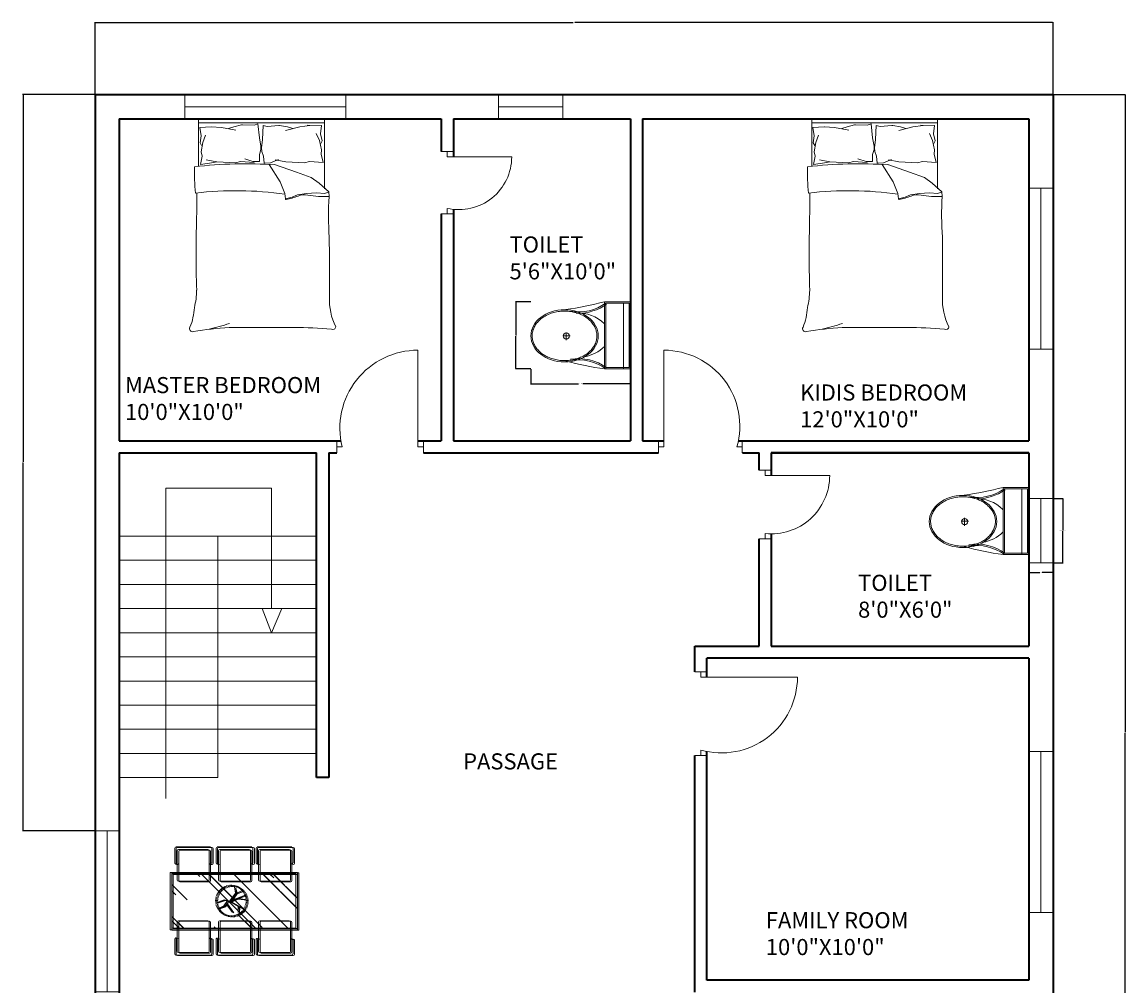
# Model space of a CAD drawing. Units: inches. Extents: x 1912 to 3731, y 1384 to 2459.
# Tile 4 of 8: x 2407 to 2818, y 1641 to 2000. Entities that reach past the tile are written whole.
import ezdxf

# ---------------------------------------------------------------- set-up
doc = ezdxf.new("R2010")
doc.units = ezdxf.units.IN
for name, color, linetype, lineweight in [('A-ANNO-DIMS', 2, 'Continuous', 18), ('A-AREA-IDEN', 7, 'Continuous', 18), ('A-DOOR', 3, 'Continuous', 20), ('A-FLOR-FIXT', 9, 'Continuous', 18), ('A-FLOR-STRS', 7, 'Continuous', 18), ('A-FURN', 8, 'Continuous', 15), ('A-GLAZ', 4, 'Continuous', 18), ('A-WALL', 7, 'Continuous', 35)]:
    doc.layers.add(name, color=color, linetype=linetype, lineweight=lineweight)
doc.styles.get("Standard").update_dxf_attribs({"font": 'arial.ttf'})
doc.dimstyles.get("Standard").update_dxf_attribs({"dimtxt": 0.18, "dimasz": 0.18, "dimexe": 0.18, "dimexo": 0.0625, "dimgap": 0.09, "dimtad": 0, "dimtih": 1, "dimtoh": 1, "dimdec": 4, "dimzin": 0, "dimdsep": 46, "dimtxsty": 'Standard', "dimcen": 0.09, "dimadec": 0, "dimazin": 0, "dimtfac": 1, "dimtdec": 4, "dimtofl": 0, "dimtmove": 0, "dimatfit": 3, "dimfxl": 1, "dimtolj": 1, "dimtzin": 0, "dimarcsym": 0})

# ---------------------------------------------------------------- blocks, each defined once
blk = doc.blocks.new('A$C31115884')
for p, q in [((257.5, 466.4), (257.5, 523.2)), ((283.1, 497.7), (223.4, 497.7)), ((0, 200), (0, 0)), ((520, 200), (0, 200)), ((10, 190), (10, 10)), ((510, 190), (10, 190)), ((510, 10), (510, 190)), ((520, 0), (520, 200)), ((510, 54.5), (0, 54.5)), ((10, 10), (510, 10)), ((0, 0), (520, 0))]:
    blk.add_line(p, q)
blk.add_circle((255.6, 496.4), 23.6)
for centre, radius, start, end in [((2777.7, -204.6), 2807, 165.4549, 171.71327), ((-294.5, 403.3), 364.7, 324.20913, 9.34987), ((-294.5, 403.3), 374.7, 324.20913, 9.34987), ((805.8, 403.3), 364.7, 170.65013, 215.79087), ((3237, 905), 2807, 188.28673, 194.5451), ((383.6, 406.2), 293.5, 190.27735, 224.15636), ((139.5, 406.2), 293.5, 315.84364, 2.65635), ((805.8, 403.3), 374.7, 179.20365, 215.79087)]:
    blk.add_arc(centre, radius, start, end)
blk.add_ellipse((256.2, 509.9), major_axis=(0, -260.7), ratio=0.772727)
blk.add_open_spline([(256.2, 259.2), (263.1, 259.2), (270, 259.7), (287.8, 262.3), (298.7, 265.1), (319.9, 273.1), (330.2, 278.4), (350.1, 291.1), (359.7, 298.7), (377.7, 315.9), (386.2, 325.5), (401.7, 346.6), (408.8, 358.1), (421.3, 382.5), (426.8, 395.5), (435.9, 422.4), (439.5, 436.4), (444.8, 465.1), (446.5, 479.7), (447.9, 509.2), (447.6, 524), (445, 553.3), (442.7, 567.8), (436.3, 596), (432.1, 609.7), (421.9, 636), (416, 648.6), (402.5, 672.1), (395, 683), (378.6, 703), (369.8, 712.1), (351.1, 728), (341.3, 734.8), (320.9, 746.2), (310.4, 750.7), (288.9, 757.3), (278, 759.4), (256, 761), (245, 760.6), (223.1, 757.2), (212.3, 754.3), (191.1, 746.1), (180.8, 740.7), (160.9, 727.8), (151.4, 720.1), (133.5, 702.7), (125.1, 693), (109.6, 671.7), (102.6, 660.2), (90.2, 635.7), (84.9, 622.7), (76, 595.6), (72.4, 581.6), (67.2, 552.9), (65.6, 538.2), (64.4, 508.8), (64.8, 494), (67.5, 464.7), (69.9, 450.2), (76.6, 422), (80.8, 408.3), (91.1, 382.2), (97.2, 369.7), (110.8, 346.3), (118.4, 335.4), (134.8, 315.6), (143.7, 306.7), (162.4, 290.9), (172.3, 284.2), (192.8, 273), (203.3, 268.6), (224.8, 262.2), (235.8, 260.2), (249.9, 259.3), (253, 259.2), (256.2, 259.2)], degree=3, knots=[0, 0, 0, 0, 0.110105, 0.110105, 0.285049, 0.285049, 0.459994, 0.459994, 0.634938, 0.634938, 0.809882, 0.809882, 0.984827, 0.984827, 1.159771, 1.159771, 1.334715, 1.334715, 1.50966, 1.50966, 1.684604, 1.684604, 1.859549, 1.859549, 2.034493, 2.034493, 2.209437, 2.209437, 2.384382, 2.384382, 2.559326, 2.559326, 2.73427, 2.73427, 2.909215, 2.909215, 3.084159, 3.084159, 3.259103, 3.259103, 3.434048, 3.434048, 3.608992, 3.608992, 3.783936, 3.783936, 3.958881, 3.958881, 4.133825, 4.133825, 4.30877, 4.30877, 4.483714, 4.483714, 4.658658, 4.658658, 4.833603, 4.833603, 5.008547, 5.008547, 5.183491, 5.183491, 5.358436, 5.358436, 5.53338, 5.53338, 5.708324, 5.708324, 5.883269, 5.883269, 6.058213, 6.058213, 6.233158, 6.233158, 6.283185, 6.283185, 6.283185, 6.283185])
blk = doc.blocks.new('BED-DOUBLE')
for p, q in [((3.41, 61.57), (3.41, 79.35)), ((3.41, 79.35), (50.34, 79.35)), ((50.34, 79.35), (50.34, 53.22)), ((3.41, 77.85), (50.34, 77.85)), ((3.82, 76.1), (4.39, 72.97)), ((3.83, 76.07), (8.03, 76.4)), ((8.03, 76.4), (8.14, 76.38)), ((8.14, 76.38), (11.89, 76.1)), ((11.89, 76.1), (17.29, 75.1)), ((14.59, 75.67), (16.58, 76.38)), ((16.58, 76.38), (19.41, 77.09)), ((19.41, 77.09), (19.73, 77.09)), ((19.73, 77.09), (24.1, 76.95)), ((24.1, 76.95), (25.52, 77.52)), ((25.52, 77.52), (26.08, 72.26)), ((27.47, 76.9), (27.24, 71.63)), ((28.93, 76.43), (27.47, 76.9)), ((33.27, 76.84), (28.93, 76.43)), ((33.59, 76.86), (33.27, 76.84)), ((36.47, 76.33), (33.59, 76.86)), ((41.16, 76.34), (35.84, 75.01)), ((38.5, 75.74), (36.47, 76.33)), ((44.89, 76.86), (41.16, 76.34)), ((49.21, 76.84), (43.91, 76.94)), ((43.91, 76.94), (44.89, 76.86)), ((49.21, 76.84), (48.84, 73.69)), ((4.39, 72.97), (3.97, 70.42)), ((3.97, 70.42), (4.53, 69.42)), ((4.39, 67.01), (4.96, 70.56)), ((4.96, 70.56), (5.95, 73.26)), ((26.08, 72.26), (26.65, 69.14)), ((27.24, 71.63), (26.86, 68.47)), ((48.42, 71.24), (47.26, 73.87)), ((49.21, 67.74), (48.42, 71.24)), ((48.84, 73.69), (49.42, 71.16)), ((49.42, 71.16), (48.92, 70.14)), ((4.68, 65.45), (4.39, 67.01)), ((26.65, 67.86), (26.08, 66.01)), ((26.08, 66.01), (26.08, 63.38)), ((26.65, 69.14), (26.65, 67.86)), ((26.86, 68.47), (26.94, 67.2)), ((26.94, 67.2), (27.62, 65.39)), ((49.03, 66.16), (49.21, 67.74)), ((49.79, 63.08), (49.03, 66.16)), ((4.11, 62.32), (4.68, 65.45)), ((9.11, 63.03), (4.11, 62.32)), ((6.27, 64), (10.23, 63.35)), ((10.23, 63.35), (9.11, 63.03)), ((10.23, 63.35), (17.11, 62.93)), ((17.11, 62.93), (19.04, 63.47)), ((19.04, 63.47), (24.08, 63.08)), ((23.67, 63.38), (20.58, 64.45)), ((26.08, 63.38), (23.67, 63.38)), ((27.62, 65.39), (27.79, 62.76)), ((27.79, 62.76), (30.2, 62.91)), ((29.72, 62.28), (33.83, 55.9)), ((30.2, 62.91), (33.21, 64.17)), ((39.91, 59.4), (31.73, 62.28)), ((31.98, 64), (35.94, 63.35)), ((35.94, 63.35), (42.82, 62.93)), ((42.82, 62.93), (44.75, 63.47)), ((44.75, 63.47), (49.79, 63.08)), ((45.39, 57.42), (39.91, 59.4)), ((33.83, 55.9), (35.5, 51.5)), ((48.28, 55.3), (45.39, 57.42)), ((51.92, 52.1), (48.28, 55.3)), ((35.5, 51.5), (35.81, 49.52)), ((35.81, 49.52), (38.24, 50.13)), ((38.24, 50.13), (40.22, 51.04)), ((40.22, 51.04), (43.56, 51.5)), ((43.56, 51.5), (47.37, 51.8)), ((47.37, 51.8), (50.41, 51.5)), ((50.41, 51.5), (51.92, 52.1)), ((52, 50.39), (51.92, 52.1, 3.8)), ((14.79, 1.53), (38.96, 1.53))]:
    blk.add_line(p, q)
for centre, radius, start, end in [((20.98, -99.43), 162, 86.0865, 96.7821), ((83.63, 59.62), 81.81, 178.7218, 185.604), ((17.44, -74.15), 126.7, 81.7845, 96.9006), ((-164.3, 48.74), 167.05, 358.4762, 1.0082), ((35.98, 49.46), 0.181, 160.2464, 271.1377), ((30.59, 77.9), 29.12, 280.6617, 289.8806), ((42.96, 44.92), 6.11, 78.6608, 113.7384), ((50.4, 85.89), 35.53, 259.8763, 272.5657), ((178.99, 43.69), 127.17, 176.9791, 183.8365), ((476.11, 29.65), 473.64, 178.2277, 181.7185), ((-4427.7, 12.75), 4479.86, 0.00217, 0.28689), ((-26.42, 16), 29.1, 346.0648, 358.9113), ((74.79, 11.92), 22.65, 177.4714, 206.4681), ((-21.27, 10.34), 23.14, 337.9751, 356.652), ((1.07, 1.07), 1.07, 146.1736, 293.4781), ((21.04, -117.88), 119.57, 92.9958, 99.4091), ((-16.91, 102.64), 104.55, 283.3832, 287.7053), ((40.41, -129.11), 130.65, 84.4998, 90.6351), ((53.43, 1.9), 1.08, 242.6588, 356.02)]:
    blk.add_arc(centre, radius, start, end)
blk = doc.blocks.new('DINING-SET-6')
h = blk.add_hatch()
h.set_pattern_fill('AR-RROOF', color=256, scale=14.228383, angle=-45, style=0)
h.set_pattern_definition([(315, (468.26, 1216.031), (32.19516, -12.07318), [213.4257, -28.4568, 71.1419, -14.2284]), (315, (486.671, 1207.68), (3.32013, 23.4421), [42.68515, -4.6954, 85.3703, -10.6713]), (315, (481.842, 1219.553), (59.05799, -45.57627), [113.82706, -19.91974, 56.9135, -14.2284])])
h.paths.add_polyline_path([(0.59, 10.06), (46.84, 10.06), (46.84, 30.22), (0.59, 30.22)])
for p, q in [((1.68, 34.33), (1.68, 39.85)), ((2.11, 40.28), (15.01, 40.28)), ((2.63, 38.9), (2.63, 27.95)), ((3.06, 39.33), (14.06, 39.33)), ((14.49, 38.9), (14.49, 27.95)), ((15.44, 39.85), (15.44, 34.33)), ((17.07, 34.33), (17.07, 39.85)), ((17.49, 40.28), (30.39, 40.28)), ((18.01, 38.9), (18.01, 27.95)), ((18.44, 39.33), (29.45, 39.33)), ((29.87, 38.9), (29.87, 27.95)), ((30.82, 39.85), (30.82, 34.33)), ((31.99, 39.85), (31.99, 34.33)), ((45.32, 40.28), (32.42, 40.28)), ((32.94, 38.9), (32.94, 27.95)), ((44.37, 39.33), (33.37, 39.33)), ((44.8, 38.9), (44.8, 27.95)), ((45.75, 34.33), (45.75, 39.85)), ((2.11, 33.9), (2.2, 33.9)), ((14.91, 33.9), (15.01, 33.9)), ((17.49, 33.9), (17.59, 33.9)), ((30.3, 33.9), (30.39, 33.9)), ((32.51, 33.9), (32.42, 33.9)), ((45.32, 33.9), (45.22, 33.9)), ((47.43, 30.81), (0, 30.81)), ((0, 30.81), (0, 9.47)), ((46.84, 30.22), (0.59, 30.22)), ((0.59, 30.22), (0.59, 10.06)), ((46.84, 10.06), (46.84, 30.22)), ((47.43, 9.47), (47.43, 30.81)), ((3.06, 27.52), (14.06, 27.52)), ((18.44, 27.52), (29.45, 27.52)), ((19.26, 24.45), (18.96, 24.82)), ((19.6, 24.7), (19.33, 25.09)), ((19.97, 24.93), (19.73, 25.34)), ((20.34, 25.13), (20.14, 25.56)), ((20.74, 25.3), (20.57, 25.74)), ((21.14, 25.44), (21.01, 25.89)), ((21.56, 25.54), (21.46, 26)), ((21.98, 25.61), (21.92, 26.08)), ((22.41, 25.65), (22.38, 26.13)), ((22.84, 25.66), (22.85, 26.13)), ((23.26, 25.63), (23.31, 26.1)), ((23.69, 25.57), (23.77, 26.03)), ((23.93, 25.25), (24.31, 23.05)), ((24.4, 23.13), (23.93, 25.25)), ((24.11, 25.47), (24.23, 25.93)), ((24.51, 25.34), (24.67, 25.79)), ((24.91, 25.18), (25.1, 25.62)), ((25.3, 25), (25.52, 25.41)), ((25.66, 24.78), (25.92, 25.17)), ((26.01, 24.53), (26.3, 24.9)), ((44.37, 27.52), (33.37, 27.52)), ((17.26, 20.78), (16.79, 20.83)), ((17.33, 21.2), (16.86, 21.29)), ((17.42, 21.62), (16.96, 21.75)), ((20.08, 20.59), (17.07, 19.53)), ((17.55, 22.03), (17.1, 22.19)), ((17.71, 22.43), (17.27, 22.62)), ((17.9, 22.81), (17.48, 23.04)), ((18.12, 23.18), (17.72, 23.44)), ((18.36, 23.53), (17.99, 23.82)), ((18.64, 23.86), (18.29, 24.18)), ((18.94, 24.17), (18.61, 24.51)), ((22.07, 20.12), (20.08, 20.59)), ((24.31, 23.05), (22.07, 20.08)), ((27.87, 22.37), (22.07, 20.08)), ((22.32, 19.95), (24.82, 21.04)), ((22.36, 20.12), (24.44, 23.05)), ((26.51, 23.81), (24.4, 23.13)), ((24.44, 23.05), (26.51, 23.81)), ((28.08, 20.67), (24.82, 21.04)), ((25.04, 21.14), (27.87, 22.37)), ((25.04, 21.14), (28.08, 20.67)), ((26.34, 24.25), (26.66, 24.61)), ((26.65, 23.95), (26.99, 24.28)), ((26.93, 23.63), (27.3, 23.93)), ((27.19, 23.29), (27.58, 23.56)), ((27.41, 22.93), (27.83, 23.16)), ((27.61, 22.55), (28.04, 22.75)), ((27.78, 22.15), (28.22, 22.32)), ((27.92, 21.75), (28.37, 21.88)), ((28.02, 21.33), (28.49, 21.43)), ((28.1, 20.91), (28.57, 20.97)), ((17.24, 20.35), (16.76, 20.37)), ((17.24, 19.93), (16.77, 19.9)), ((17.28, 19.5), (16.81, 19.44)), ((17.35, 19.08), (16.89, 18.98)), ((17.46, 18.66), (17, 18.53)), ((17.07, 19.53), (20.08, 20.46)), ((17.59, 18.26), (17.15, 18.09)), ((17.76, 17.86), (17.33, 17.66)), ((17.96, 17.48), (17.55, 17.25)), ((18.19, 17.12), (17.8, 16.85)), ((20.03, 18.3), (18, 17.37)), ((18, 17.37), (20.16, 18.21)), ((18.45, 16.78), (18.08, 16.48)), ((21.3, 20.29), (20.03, 18.3)), ((20.08, 20.46), (22.32, 19.91)), ((20.16, 18.21), (21.35, 20.16)), ((23.21, 15.88), (20.71, 19.23)), ((20.84, 19.23), (23.21, 15.88)), ((25.33, 18.16), (22.11, 19.91)), ((22.36, 19.95), (27.32, 17.07)), ((25.33, 15.84), (25.33, 18.16)), ((25.43, 18.1), (25.33, 15.84)), ((27.32, 17.07), (25.43, 18.1)), ((26.74, 16.55), (27.09, 16.23)), ((27.01, 16.88), (27.39, 16.59)), ((27.26, 17.23), (27.66, 16.97)), ((27.48, 17.6), (27.89, 17.37)), ((27.67, 17.98), (28.1, 17.79)), ((27.83, 18.38), (28.27, 18.22)), ((27.95, 18.79), (28.41, 18.66)), ((28.05, 19.2), (28.52, 19.12)), ((28.11, 19.63), (28.58, 19.58)), ((28.13, 20.48), (28.61, 20.51)), ((28.14, 20.06), (28.61, 20.04)), ((3.06, 12.76), (14.06, 12.76)), ((18.73, 16.45), (18.38, 16.13)), ((18.44, 12.76), (29.45, 12.76)), ((19.03, 16.16), (18.72, 15.8)), ((19.36, 15.88), (19.07, 15.51)), ((19.71, 15.63), (19.45, 15.24)), ((20.08, 15.41), (19.85, 15)), ((20.46, 15.22), (20.27, 14.79)), ((20.86, 15.07), (20.7, 14.62)), ((21.27, 14.94), (21.15, 14.48)), ((21.69, 14.84), (21.6, 14.38)), ((22.11, 14.78), (22.06, 14.31)), ((22.54, 14.75), (22.53, 14.28)), ((22.97, 14.76), (22.99, 14.28)), ((23.39, 14.8), (23.46, 14.33)), ((23.82, 14.87), (23.91, 14.4)), ((24.23, 14.97), (24.37, 14.52)), ((24.64, 15.11), (24.81, 14.67)), ((25.03, 15.28), (25.23, 14.85)), ((25.41, 15.48), (25.65, 15.07)), ((25.77, 15.71), (26.04, 15.32)), ((26.12, 15.96), (26.41, 15.59)), ((26.44, 16.24), (26.76, 15.9)), ((44.37, 12.76), (33.37, 12.76)), ((0, 9.47), (47.43, 9.47)), ((0.59, 10.06), (46.84, 10.06)), ((2.63, 12.33), (2.63, 1.38)), ((14.49, 1.38), (14.49, 12.33)), ((18.01, 12.33), (18.01, 1.38)), ((29.87, 1.38), (29.87, 12.33)), ((32.94, 1.38), (32.94, 12.33)), ((44.8, 12.33), (44.8, 1.38)), ((1.68, 5.95), (1.68, 0.43)), ((2.11, 6.38), (2.21, 6.38)), ((14.92, 6.29), (15.01, 6.29)), ((15.44, 0.43), (15.44, 5.95)), ((17.07, 5.95), (17.07, 0.43)), ((17.5, 6.27), (17.59, 6.27)), ((30.3, 6.19), (30.4, 6.19)), ((30.82, 0.43), (30.82, 5.95)), ((31.99, 0.43), (31.99, 5.95)), ((32.52, 6.17), (32.42, 6.18)), ((45.32, 6.09), (45.23, 6.09)), ((45.75, 5.95), (45.75, 0.43)), ((3.06, 0.95), (14.06, 0.95)), ((18.44, 0.95), (29.45, 0.95)), ((44.37, 0.95), (33.37, 0.95)), ((2.11, 0), (15.01, 0)), ((17.49, 0), (30.39, 0)), ((45.32, 0), (32.42, 0))]:
    blk.add_line(p, q)
for centre, start, end in [((2.11, 39.85), 90, 180), ((3.06, 38.9), 90, 180), ((14.06, 38.9), 0, 90), ((15.01, 39.85), 0, 90), ((17.49, 39.85), 90, 180), ((18.44, 38.9), 90, 180), ((29.45, 38.9), 0, 90), ((30.39, 39.85), 0, 90), ((32.42, 39.85), 90, 180), ((33.37, 38.9), 90, 180), ((44.37, 38.9), 0, 90), ((45.32, 39.85), 0, 90), ((2.11, 34.33), 180, 0.104), ((14.91, 34.33), 180, 0.104), ((17.49, 34.33), 180, 270), ((17.59, 34.33), 270, 0), ((30.3, 34.33), 180, 270), ((30.39, 34.33), 270, 0), ((32.42, 34.33), 180, 270), ((32.51, 34.33), 270, 0), ((45.22, 34.33), 180, 270), ((45.32, 34.33), 270, 0), ((3.06, 27.95), 180, 270), ((14.06, 27.95), 270, 0), ((18.44, 27.95), 180, 270), ((29.45, 27.95), 270, 0), ((33.37, 27.95), 180, 270), ((44.37, 27.95), 270, 0), ((3.06, 12.33), 90, 180), ((14.06, 12.33), 0, 90), ((18.44, 12.33), 90, 180), ((29.45, 12.33), 0, 90), ((33.37, 12.33), 90, 180), ((44.37, 12.33), 0, 90), ((2.11, 5.95), 89.6202, 179.6202), ((2.2, 5.95), 359.6202, 89.6202), ((14.91, 5.86), 89.6202, 179.6202), ((15.01, 5.86), 359.6202, 89.6202), ((17.49, 5.85), 89.6202, 179.6202), ((17.59, 5.85), 359.6202, 89.6202), ((30.3, 5.76), 89.6202, 179.6202), ((30.39, 5.76), 359.6202, 89.6202), ((32.42, 5.75), 89.6202, 179.6202), ((32.51, 5.75), 359.6202, 89.6202), ((45.22, 5.66), 89.6202, 179.6202), ((45.32, 5.66), 359.6202, 89.6202), ((2.11, 0.43), 180, 270), ((3.06, 1.38), 180, 270), ((14.06, 1.38), 270, 0), ((15.01, 0.43), 270, 0), ((17.49, 0.43), 180, 270), ((18.44, 1.38), 180, 270), ((29.45, 1.38), 270, 0), ((30.39, 0.43), 270, 0), ((32.42, 0.43), 180, 270), ((33.37, 1.38), 180, 270), ((44.37, 1.38), 270, 0), ((45.32, 0.43), 270, 0)]:
    blk.add_arc(centre, 0.427, start, end)
blk = doc.blocks.new('STAIR-RETURN-FIRST')
for p, q in [((17.33, 0), (17.33, 115.73)), ((17.33, 115.73), (56.7, 115.73)), ((56.7, 115.73), (56.7, 70.82)), ((36.78, 97.82), (0, 97.82)), ((36.78, 7.82), (36.78, 97.82)), ((36.78, 97.82), (73.56, 97.82)), ((36.78, 88.82), (0, 88.82)), ((36.78, 88.82), (73.56, 88.82)), ((36.78, 79.82), (0, 79.82)), ((36.78, 79.82), (73.56, 79.82)), ((36.78, 70.82), (0, 70.82)), ((36.78, 70.82), (73.56, 70.82)), ((60.6, 70.82), (53.28, 70.82)), ((53.28, 70.82), (56.7, 61.82)), ((56.7, 61.82), (60.6, 70.82)), ((36.78, 61.82), (0, 61.82)), ((36.78, 61.82), (73.56, 61.82)), ((36.78, 52.82), (0, 52.82)), ((36.78, 52.82), (73.56, 52.82)), ((36.78, 43.82), (0, 43.82)), ((36.78, 43.82), (73.56, 43.82)), ((36.78, 34.82), (0, 34.82)), ((36.78, 34.82), (73.56, 34.82)), ((36.78, 25.82), (0, 25.82)), ((36.78, 25.82), (73.56, 25.82)), ((36.78, 16.82), (0, 16.82)), ((36.78, 7.82), (36.78, 16.82)), ((36.78, 16.82), (73.56, 16.82)), ((36.78, 7.82), (0, 7.82))]:
    blk.add_line(p, q)
blk = doc.blocks.new('DOOR-24-FF-ENSUITE')
for p, q in [((0, 23.22), (4.5, 23.22)), ((4.5, 23.22), (2.25, 23.22)), ((2.25, 23.22), (2.25, 21.22)), ((2.25, 21.22), (26.25, 21.22)), ((0, 0), (4.5, 0)), ((2.25, 0), (2.25, 2)), ((4.5, 0), (2.25, 0))]:
    blk.add_line(p, q)
blk.add_arc((6.56, 21.22), 19.69, 257.3694, 0)
blk = doc.blocks.new('DOOR-36-FF-MASTER')
for p, q in [((30.28, 2.25), (30.28, 38.25)), ((0, 4.5), (0, 0)), ((32.28, 4.5), (32.28, 0)), ((0, 0), (0, 2.25)), ((0, 2.25), (2, 2.25)), ((32.28, 2.25), (30.28, 2.25)), ((32.28, 0), (32.28, 2.25))]:
    blk.add_line(p, q)
blk.add_arc((30.28, 9.14), 29.11, 90, 193.7017)
blk = doc.blocks.new('DOOR-36-FF-KIDS')
for p, q in [((2, 2.25), (2, 38.25)), ((0, 4.5), (0, 0)), ((31.21, 4.5), (31.21, 0)), ((0, 0), (0, 2.25)), ((0, 2.25), (2, 2.25)), ((31.21, 2.25), (29.21, 2.25)), ((31.21, 0), (31.21, 2.25))]:
    blk.add_line(p, q)
blk.add_arc((2, 9.97), 28.28, 344.169, 90)
blk = doc.blocks.new('DOOR-24-FF-BATH')
for p, q in [((0, 25.59), (4.5, 25.59)), ((4.5, 25.59), (0, 25.59)), ((0, 25.59), (2.25, 25.59)), ((2.25, 25.59), (2.25, 23.59)), ((2.25, 23.59), (26.25, 23.59)), ((2.25, 0), (2.25, 2)), ((0, 0), (4.5, 0)), ((4.5, 0), (2.25, 0))]:
    blk.add_line(p, q)
blk.add_arc((4.54, 23.59), 21.71, 263.9539, 0)
blk = doc.blocks.new('DOOR-36-FF-FAMILY')
for p, q in [((4.5, 31.2), (0, 31.2)), ((0, 31.2), (2.25, 31.2)), ((2.25, 31.2), (2.25, 29.2)), ((2.25, 29.2), (38.25, 29.2)), ((2.25, 0), (2.25, 2)), ((0, 0), (4.5, 0)), ((4.5, 0), (2.25, 0))]:
    blk.add_line(p, q)
blk.add_arc((9.98, 29.2), 28.27, 254.1384, 0)
blk = doc.blocks.new('WIN-PLAN-60-A')
for p, q in [((0, 9), (0, 0)), ((60, 4.5), (60, 9)), ((60, 9), (60, 0)), ((0, 0), (0, 4.5)), ((0, 4.5), (60, 4.5))]:
    blk.add_line(p, q)
blk = doc.blocks.new('WIN-PLAN-60-B')
for p, q in [((0, 60), (9, 60)), ((9, 60), (4.5, 60)), ((4.5, 60), (4.5, 0)), ((9, 0), (0, 0)), ((4.5, 0), (9, 0))]:
    blk.add_line(p, q)
blk = doc.blocks.new('WIN-PLAN-24-A')
for p, q in [((0, 24), (9, 24)), ((9, 24), (4.5, 24)), ((4.5, 24), (4.5, 0)), ((4.5, 0), (0, 0)), ((0, 0), (9, 0))]:
    blk.add_line(p, q)
blk = doc.blocks.new('WIN-PLAN-24-B')
for p, q in [((0, 24), (9, 24)), ((9, 24), (4.5, 24)), ((4.5, 24), (4.5, 0)), ((9, 0), (0, 0)), ((4.5, 0), (9, 0))]:
    blk.add_line(p, q)
blk = doc.blocks.new('WIN-PLAN-60-C')
for p, q in [((0, 9), (0, 0)), ((60, 4.5), (60, 9)), ((60, 9), (60, 0)), ((0, 4.5), (60, 4.5))]:
    blk.add_line(p, q)
blk = doc.blocks.new('*D37')
at = {"layer": 'A-ANNO-DIMS', "color": 0, "lineweight": -2, "transparency": 16777216}
for p, q in [((2791.37, 1822.63), (2795.09, 1822.63)), ((2794.91, 1822.45), (2794.91, 1810.81)), ((2794.91, 1798.81), (2794.91, 1810.45)), ((2791.37, 1798.63), (2795.09, 1798.63))]:
    blk.add_line(p, q, dxfattribs=at)
at = {"layer": 'A-ANNO-DIMS', "color": 0, "transparency": 16777216}
for points in [[(2794.88, 1822.45), (2794.94, 1822.45), (2794.91, 1822.63)], [(2794.88, 1798.81), (2794.94, 1798.81), (2794.91, 1798.63)]]:
    blk.add_solid(points, dxfattribs=at)
at = {"layer": 'Defpoints', "color": 0, "transparency": 16777216}
for p in [(2791.31, 1822.63), (2794.91, 1822.63), (2791.31, 1798.63)]:
    blk.add_point(p, dxfattribs=at)
at = {"layer": 'A-ANNO-DIMS', "color": 0, "transparency": 16777216, "insert": (2794.91, 1810.63), "char_height": 0.18, "attachment_point": 5}
blk.add_mtext('\\A1;WC WINDOW 24 TYP.', dxfattribs=at)
blk = doc.blocks.new('*D38')
at = {"layer": 'A-ANNO-DIMS', "color": 0, "lineweight": -2, "transparency": 16777216}
for p, q in [((2782.31, 1798.57), (2782.31, 1794.85)), ((2791.31, 1798.57), (2791.31, 1794.85)), ((2782.49, 1795.03), (2786.35, 1795.03)), ((2791.13, 1795.03), (2787.27, 1795.03))]:
    blk.add_line(p, q, dxfattribs=at)
at = {"layer": 'A-ANNO-DIMS', "color": 0, "transparency": 16777216}
for points in [[(2782.49, 1795.06), (2782.49, 1795), (2782.31, 1795.03)], [(2791.13, 1795.06), (2791.13, 1795), (2791.31, 1795.03)]]:
    blk.add_solid(points, dxfattribs=at)
at = {"layer": 'Defpoints', "color": 0, "transparency": 16777216}
for p in [(2782.31, 1798.63), (2791.31, 1798.63), (2791.31, 1795.03)]:
    blk.add_point(p, dxfattribs=at)
at = {"layer": 'A-ANNO-DIMS', "color": 0, "transparency": 16777216, "insert": (2786.81, 1795.03), "char_height": 0.18, "attachment_point": 5}
blk.add_mtext('\\A1;9 TYP.', dxfattribs=at)
blk = doc.blocks.new('*D61')
at = {"layer": 'A-ANNO-DIMS', "color": 0, "lineweight": -2, "transparency": 16777216}
for p, q in [((2596.7, 1870.82), (2596.7, 1865.14)), ((2633.81, 1870.82), (2633.81, 1865.14)), ((2596.88, 1865.32), (2614.48, 1865.32)), ((2633.63, 1865.32), (2616.03, 1865.32))]:
    blk.add_line(p, q, dxfattribs=at)
at = {"layer": 'A-ANNO-DIMS', "color": 0, "transparency": 16777216}
for points in [[(2596.88, 1865.35), (2596.88, 1865.29), (2596.7, 1865.32)], [(2633.63, 1865.35), (2633.63, 1865.29), (2633.81, 1865.32)]]:
    blk.add_solid(points, dxfattribs=at)
at = {"layer": 'Defpoints', "color": 0, "transparency": 16777216}
for p in [(2596.7, 1870.89), (2633.81, 1870.89), (2596.7, 1865.32)]:
    blk.add_point(p, dxfattribs=at)
at = {"layer": 'A-ANNO-DIMS', "color": 0, "transparency": 16777216, "insert": (2615.25, 1865.32), "char_height": 0.18, "attachment_point": 5}
blk.add_mtext('\\A1;WC 37 TYP.', dxfattribs=at)
blk = doc.blocks.new('*D62')
at = {"layer": 'A-ANNO-DIMS', "color": 0, "lineweight": -2, "transparency": 16777216}
for p, q in [((2596.63, 1895.93), (2590.95, 1895.93)), ((2591.13, 1895.75), (2591.13, 1883.59)), ((2591.13, 1871.07), (2591.13, 1883.23)), ((2596.63, 1870.89), (2590.95, 1870.89))]:
    blk.add_line(p, q, dxfattribs=at)
at = {"layer": 'A-ANNO-DIMS', "color": 0, "transparency": 16777216}
for points in [[(2591.1, 1895.75), (2591.16, 1895.75), (2591.13, 1895.93)], [(2591.1, 1871.07), (2591.16, 1871.07), (2591.13, 1870.89)]]:
    blk.add_solid(points, dxfattribs=at)
at = {"layer": 'Defpoints', "color": 0, "transparency": 16777216}
for p in [(2591.13, 1895.93), (2596.7, 1895.93), (2596.7, 1870.89)]:
    blk.add_point(p, dxfattribs=at)
at = {"layer": 'A-ANNO-DIMS', "color": 0, "transparency": 16777216, "insert": (2591.13, 1883.41), "char_height": 0.18, "attachment_point": 5}
blk.add_mtext('\\A1;25 TYP.', dxfattribs=at)
blk = doc.blocks.new('*D99')
at = {"layer": 'A-ANNO-DIMS', "color": 0, "lineweight": -2, "transparency": 16777216}
for p, q in [((2434.31, 1973.19), (2434.31, 2000.16)), ((2434.49, 1999.98), (2612.52, 1999.98)), ((2791.13, 1999.98), (2613.1, 1999.98)), ((2791.31, 1973.19), (2791.31, 2000.16))]:
    blk.add_line(p, q, dxfattribs=at)
at = {"layer": 'A-ANNO-DIMS', "color": 0, "transparency": 16777216}
for points in [[(2434.49, 2000.01), (2434.49, 1999.95), (2434.31, 1999.98)], [(2791.13, 2000.01), (2791.13, 1999.95), (2791.31, 1999.98)]]:
    blk.add_solid(points, dxfattribs=at)
at = {"layer": 'Defpoints', "color": 0, "transparency": 16777216}
for p in [(2791.31, 1999.98), (2434.31, 1973.13), (2791.31, 1973.13)]:
    blk.add_point(p, dxfattribs=at)
at = {"layer": 'A-ANNO-DIMS', "color": 0, "transparency": 16777216, "insert": (2612.81, 1999.98), "char_height": 0.18, "attachment_point": 5}
blk.add_mtext('\\A1;357', dxfattribs=at)
blk = doc.blocks.new('*D100')
at = {"layer": 'A-ANNO-DIMS', "color": 0, "lineweight": -2, "transparency": 16777216}
for p, q in [((2791.37, 1973.13), (2818.34, 1973.13)), ((2818.16, 1972.95), (2818.16, 1735.56)), ((2818.16, 1497.81), (2818.16, 1735.19)), ((2791.37, 1497.63), (2818.34, 1497.63))]:
    blk.add_line(p, q, dxfattribs=at)
at = {"layer": 'A-ANNO-DIMS', "color": 0, "transparency": 16777216}
for points in [[(2818.13, 1972.95), (2818.19, 1972.95), (2818.16, 1973.13)], [(2818.13, 1497.81), (2818.19, 1497.81), (2818.16, 1497.63)]]:
    blk.add_solid(points, dxfattribs=at)
at = {"layer": 'Defpoints', "color": 0, "transparency": 16777216}
for p in [(2791.31, 1973.13), (2818.16, 1973.13), (2791.31, 1497.63)]:
    blk.add_point(p, dxfattribs=at)
at = {"layer": 'A-ANNO-DIMS', "color": 0, "transparency": 16777216, "insert": (2818.16, 1735.38), "char_height": 0.18, "attachment_point": 5}
blk.add_mtext('\\A1;475.5', dxfattribs=at)
blk = doc.blocks.new('*D101')
at = {"layer": 'A-ANNO-DIMS', "color": 0, "lineweight": -2, "transparency": 16777216}
for p, q in [((2434.25, 1973.13), (2407.28, 1973.13)), ((2407.46, 1972.95), (2407.46, 1836.14)), ((2407.46, 1698.96), (2407.46, 1835.77)), ((2434.25, 1698.78), (2407.28, 1698.78))]:
    blk.add_line(p, q, dxfattribs=at)
at = {"layer": 'A-ANNO-DIMS', "color": 0, "transparency": 16777216}
for points in [[(2407.43, 1972.95), (2407.49, 1972.95), (2407.46, 1973.13)], [(2407.43, 1698.96), (2407.49, 1698.96), (2407.46, 1698.78)]]:
    blk.add_solid(points, dxfattribs=at)
at = {"layer": 'Defpoints', "color": 0, "transparency": 16777216}
for p in [(2434.31, 1973.13), (2407.46, 1698.78), (2434.31, 1698.78)]:
    blk.add_point(p, dxfattribs=at)
at = {"layer": 'A-ANNO-DIMS', "color": 0, "transparency": 16777216, "insert": (2407.46, 1835.95), "char_height": 0.18, "attachment_point": 5}
blk.add_mtext('\\A1;274.34', dxfattribs=at)

msp = doc.modelspace()

# ---------------------------------------------------------------- linework, layer by layer
at = {"layer": 'A-WALL'}
for p, q in [((2434.311, 1973.1258), (2434.311, 1497.6258)), ((2434.311, 1973.1258), (2791.311, 1973.1258)), ((2791.311, 1973.1258), (2791.311, 1497.6258)), ((2443.311, 1964.1258), (2563.311, 1964.1258)), ((2443.311, 1964.1258), (2443.311, 1844.1258)), ((2563.311, 1964.1258), (2563.311, 1951.9406)), ((2567.811, 1964.1258), (2567.811, 1949.9406)), ((2567.811, 1964.1258), (2633.811, 1964.1258)), ((2633.811, 1964.1258), (2633.811, 1844.1258)), ((2638.311, 1964.1258), (2638.311, 1844.1258)), ((2638.311, 1964.1258), (2782.311, 1964.1258)), ((2782.311, 1964.1258), (2782.311, 1844.1258)), ((2567.811, 1930.3545), (2567.811, 1844.1258)), ((2563.311, 1928.7235), (2563.311, 1844.1258)), ((2443.311, 1844.1258), (2525.8943, 1844.1258)), ((2554.6272, 1844.1258), (2563.311, 1844.1258)), ((2567.811, 1844.1258), (2633.811, 1844.1258)), ((2638.311, 1844.1258), (2646.301, 1844.1258)), ((2674.0519, 1844.1258), (2782.311, 1844.1258)), ((2443.311, 1839.6258), (2516.8684, 1839.6258)), ((2443.311, 1839.6258), (2443.311, 1506.6258)), ((2516.8684, 1718.5838), (2516.8684, 1839.6258)), ((2521.3684, 1839.6258), (2521.3684, 1718.5838)), ((2521.3684, 1839.6258), (2524.3497, 1839.6258)), ((2556.6272, 1839.6258), (2644.301, 1839.6258)), ((2675.5123, 1839.6258), (2681.811, 1839.6258)), ((2681.811, 1833.1769), (2681.811, 1839.6258)), ((2782.311, 1839.6258), (2686.311, 1839.6258)), ((2686.311, 1839.6258), (2686.311, 1831.1769)), ((2686.311, 1839.6258), (2782.311, 1839.6258)), ((2782.311, 1839.6258), (2782.311, 1767.6258)), ((2681.811, 1767.6258), (2681.811, 1807.5847)), ((2686.311, 1809.4639), (2686.311, 1767.6258)), ((2657.811, 1767.6258), (2681.811, 1767.6258)), ((2657.811, 1758.0661), (2657.811, 1767.6258)), ((2686.311, 1767.6258), (2782.311, 1767.6258)), ((2681.811, 1763.1258), (2662.311, 1763.1258)), ((2662.311, 1756.0661), (2662.311, 1763.1258)), ((2686.311, 1763.1258), (2681.811, 1763.1258)), ((2782.311, 1763.1258), (2686.311, 1763.1258)), ((2782.311, 1763.1258), (2782.311, 1643.1258)), ((2662.311, 1643.1258), (2662.311, 1728.3291)), ((2657.811, 1638.6258), (2657.811, 1726.8699)), ((2521.3684, 1718.5838), (2516.8684, 1718.5838)), ((2782.311, 1643.1258), (2662.311, 1643.1258)), ((2782.311, 1643.1258), (2686.311, 1643.1258))]:
    msp.add_line(p, q, dxfattribs=at)

# ---------------------------------------------------------------- block references
at = {"layer": 'A-DOOR'}
for name, p in [('DOOR-24-FF-ENSUITE', (2563.311, 1928.723)), ('DOOR-36-FF-MASTER', (2524.35, 1839.626)), ('DOOR-36-FF-KIDS', (2644.301, 1839.626)), ('DOOR-24-FF-BATH', (2681.811, 1807.585)), ('DOOR-36-FF-FAMILY', (2657.811, 1726.87))]:
    msp.add_blockref(name, p, dxfattribs=at)
at = {"layer": 'A-FLOR-FIXT', "xscale": 0.048164045903398, "yscale": 0.048164045903398, "zscale": 0.048164045903398, "rotation": 89.99999999999991}
for p in [(2633.811, 1870.8856), (2782.311, 1801.704)]:
    msp.add_blockref('A$C31115884', p, dxfattribs=at)
at = {"layer": 'A-FLOR-STRS'}
msp.add_blockref('STAIR-RETURN-FIRST', (2443.311, 1710.768), dxfattribs=at)
at = {"layer": 'A-FURN'}
for name, p in [('BED-DOUBLE', (2469.4756, 1884.774)), ('BED-DOUBLE', (2697.9527, 1884.774)), ('DINING-SET-6', (2462.3064, 1652.4494)), ('DINING-SET-6', (2462.8449, 1652.2699))]:
    msp.add_blockref(name, p, dxfattribs=at)
at = {"layer": 'A-GLAZ'}
for name, p in [('WIN-PLAN-60-C', (2467.702, 1964.126)), ('WIN-PLAN-24-B', (2782.311, 1798.63))]:
    msp.add_blockref(name, p, dxfattribs=at)
at = {"layer": 'A-GLAZ', "extrusion": (0, 0, -1), "zscale": -1, "rotation": 90}
for name, p in [('WIN-PLAN-24-A', (-2584.6491, 1964.126)), ('WIN-PLAN-60-A', (-2782.3113, 1878.2056)), ('WIN-PLAN-60-A', (-2782.3113, 1668.3249))]:
    msp.add_blockref(name, p, dxfattribs=at)
at = {"layer": 'A-GLAZ', "rotation": 180}
msp.add_blockref('WIN-PLAN-60-B', (2443.3108, 1698.7837), dxfattribs=at)

# ---------------------------------------------------------------- texts
at = {"layer": 'A-AREA-IDEN', "char_height": 6, "attachment_point": 1}
for s, width, insert in [('TOILET\\P5\'6"X10\'0"', 95.120473, (2588.7511, 1920.2715)), ('MASTER BEDROOM\\P10\'0"X10\'0"', 128.861593, (2445.4446, 1867.8697)), ('KIDIS BEDROOM\\P12\'0"X10\'0"', 115.981433, (2697.0516, 1865.1083)), ('TOILET\\P8\'0"X6\'0"', 93.474207, (2718.648, 1794.1798)), ('PASSAGE', 152.030801, (2571.457, 1727.6353)), ('FAMILY ROOM \\P10\'0"X10\'0"', 123.70951, (2684.2725, 1668.4503))]:
    msp.add_mtext_dynamic_manual_height_columns(s, width=width, gutter_width=12.5, heights=[0], dxfattribs=dict(at, insert=insert))

# ---------------------------------------------------------------- dimensions: what is measured, and where the dimension line sits
at = {"layer": 'A-ANNO-DIMS'}
dim = msp.add_linear_dim(base=(2791.311, 1999.9758), p1=(2434.311, 1973.1258), p2=(2791.311, 1973.1258), dimstyle='Standard', override={"dimdec": 0, "dimlfac": 1, "dimrnd": 0, "dimzin": 0, "dimdsep": 46, "dimlunit": 2}, dxfattribs=at)
dim.commit()
dim.dimension.update_dxf_attribs({"geometry": '*D99', "text_midpoint": (2612.811, 1999.9758)})
for base, p1, p2, override, picture, middle in [((2407.461, 1698.7838), (2434.311, 1973.1258), (2434.311, 1698.7838), {"dimdec": 2, "dimlfac": 1, "dimrnd": 0, "dimzin": 0, "dimdsep": 46, "dimlunit": 2}, '*D101', (2407.461, 1835.9548)), ((2818.161, 1973.1258), (2791.311, 1497.6258), (2791.311, 1973.1258), {"dimdec": 1, "dimlfac": 1, "dimrnd": 0, "dimzin": 0, "dimdsep": 46, "dimlunit": 2}, '*D100', (2818.161, 1735.3758))]:
    dim = msp.add_linear_dim(base=base, p1=p1, p2=p2, angle=90, dimstyle='Standard', override=override, dxfattribs=at)
    dim.commit()
    dim.dimension.update_dxf_attribs({"geometry": picture, "text_midpoint": middle})
for base, p1, p2, angle, text, picture, middle in [((2591.1302, 1895.9309), (2596.6973, 1870.8856), (2596.6973, 1895.9309), 90, '<> TYP.', '*D62', (2591.1302, 1883.4083)), ((2596.6973, 1865.3186), (2633.811, 1870.8856), (2596.6973, 1870.8856), 180, 'WC <> TYP.', '*D61', (2615.2542, 1865.3186)), ((2794.911, 1822.6304), (2791.311, 1798.6304), (2791.311, 1822.6304), 90, 'WC WINDOW <> TYP.', '*D37', (2794.911, 1810.6304))]:
    dim = msp.add_linear_dim(base=base, p1=p1, p2=p2, angle=angle, text=text, dimstyle='Standard', override={"dimdec": 0, "dimlfac": 1, "dimrnd": 0, "dimzin": 0, "dimdsep": 46, "dimlunit": 2}, dxfattribs=at)
    dim.commit()
    dim.dimension.update_dxf_attribs({"geometry": picture, "text_midpoint": middle})
dim = msp.add_linear_dim(base=(2791.311, 1795.0304), p1=(2782.311, 1798.6304), p2=(2791.311, 1798.6304), text='<> TYP.', dimstyle='Standard', override={"dimdec": 0, "dimlfac": 1, "dimrnd": 0, "dimzin": 0, "dimdsep": 46, "dimlunit": 2}, dxfattribs=at)
dim.commit()
dim.dimension.update_dxf_attribs({"geometry": '*D38', "text_midpoint": (2786.811, 1795.0304)})

doc.saveas('drawing.dxf')
